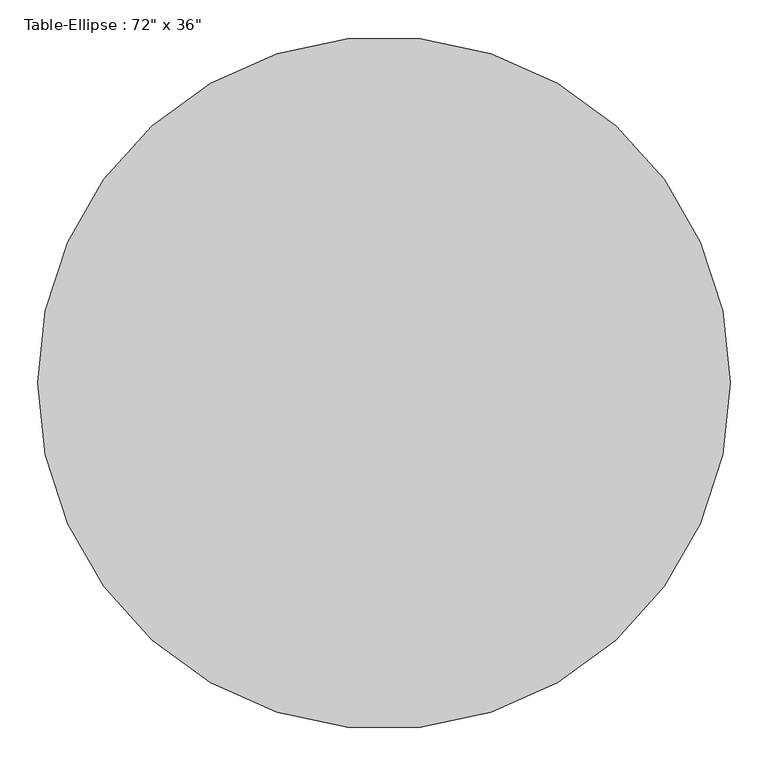
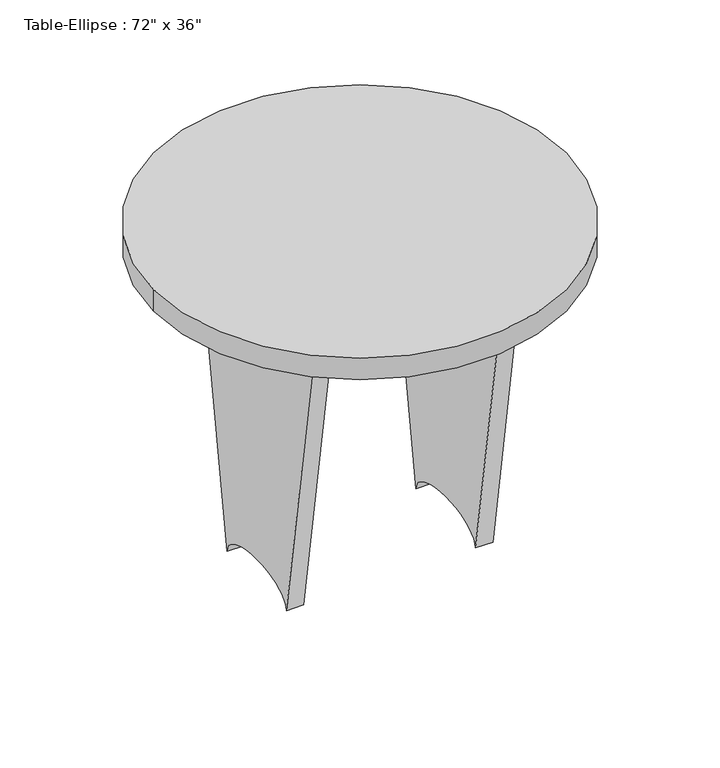
"""IFC4 building model written with IfcOpenShell, lengths in millimetres: furniture geometry."""

from ifc_helpers import new_model, si_unit, point, frame, origin, place, context, project, spatial, circle_curve, ellipse_curve, trimmed, source, transform, mapped, element, save
from ifc_brep_helpers import plane_surface, extruded_surface, advanced_brep


def furniture_4bee3317(model_context):
    return source(origin(), model_context, "Body", "AdvancedBrep", [
        advanced_brep(
        [(-190.5, 19.05, 711.2), (190.5, 19.05, 711.2), (190.5, 19.05, 474.1333333), (-190.5, 19.05, 474.1333333), (-190.5, -19.05, 711.2), (-190.5, -19.05, 474.1333333), (190.5, -19.05, 474.1333333), (190.5, -19.05, 711.2)],
        [
            (0, 1),
            (1, 2),
            (2, 3, ellipse_curve(frame((0.0, 19.05, 474.1333333), z_axis=(0.0, -1.0, 0.0), x_axis=(1.0, 0.0, 0.0)), 190.5, 101.6)),
            (3, 0),
            (4, 5),
            (5, 6, ellipse_curve(frame((0.0, -19.05, 474.1333333), z_axis=(0.0, 1.0, 0.0), x_axis=(1.0, 0.0, 0.0)), 190.5, 101.6)),
            (6, 7),
            (7, 4),
            (0, 4),
            (7, 1),
            (6, 2),
            (5, 3),
        ],
        [
            plane_surface(frame((-190.5, 19.05, 711.2), z_axis=(0.0, 1.0, 0.0), x_axis=(1.0, 0.0, 0.0))),
            plane_surface(frame((-190.5, -19.05, 711.2), z_axis=(0.0, -1.0, 0.0), x_axis=(-1.0, 0.0, 0.0))),
            plane_surface(frame((-190.5, 19.05, 711.2), z_axis=(0.0, 0.0, 1.0), x_axis=(0.0, -1.0, 0.0))),
            plane_surface(frame((190.5, 19.05, 711.2), z_axis=(1.0, 0.0, 0.0), x_axis=(0.0, -1.0, 0.0))),
            extruded_surface(trimmed(ellipse_curve(frame((0.0, -57.15, 474.1333333), z_axis=(0.0, -1.0, 0.0), x_axis=(1.0, 0.0, 0.0)), 190.5, 101.6), [point((190.5, -57.15, 474.1333333))], [point((-190.5, -57.15, 474.1333333))], True, "CARTESIAN"), (0.0, 38.099999999999994, 0.0), 38.099999999999994),
            plane_surface(frame((-190.5, 19.05, 474.1333333), z_axis=(-1.0, 0.0, 0.0), x_axis=(0.0, -1.0, 0.0))),
        ],
        [
            (0, [[1, 2, 3, 4]]),
            (1, [[5, 6, 7, 8]]),
            (2, [[-1, 9, -8, 10]]),
            (3, [[-2, -10, -7, 11]]),
            (4, [[-3, -11, -6, 12]]),
            (5, [[-4, -12, -5, -9]]),
        ],
    ),
        advanced_brep(
        [(228.6, 228.6, 711.2), (228.6, -228.6, 711.2), (228.6, -114.3, 0.0), (228.6, 114.3, 0.0), (190.5, 228.6, 711.2), (190.5, 114.3, 0.0), (190.5, -114.3, 0.0), (190.5, -228.6, 711.2)],
        [
            (0, 1),
            (1, 2),
            (2, 3, ellipse_curve(frame((228.6, 0.0, 0.0), z_axis=(-1.0, 0.0, 0.0), x_axis=(0.0, 1.0, 0.0)), 114.3, 50.8)),
            (3, 0),
            (4, 5),
            (5, 6, ellipse_curve(frame((190.5, 0.0, 0.0), z_axis=(1.0, 0.0, 0.0), x_axis=(0.0, 1.0, 0.0)), 114.3, 50.8)),
            (6, 7),
            (7, 4),
            (0, 4),
            (7, 1),
            (6, 2),
            (5, 3),
        ],
        [
            plane_surface(frame((228.6, -228.6, 711.2), z_axis=(1.0, 0.0, 0.0), x_axis=(0.0, -1.0, 0.0))),
            plane_surface(frame((190.5, -228.6, 711.2), z_axis=(-1.0, 0.0, 0.0), x_axis=(0.0, 1.0, 0.0))),
            plane_surface(frame((228.6, 228.6, 711.2), z_axis=(0.0, 0.0, 1.0), x_axis=(-1.0, 0.0, 0.0))),
            plane_surface(frame((228.6, -228.6, 711.2), z_axis=(0.0, -0.9873303712766982, -0.158678095383759), x_axis=(-1.0, 0.0, 0.0))),
            extruded_surface(trimmed(ellipse_curve(frame((152.4, 0.0, 0.0), z_axis=(-1.0, 0.0, 0.0), x_axis=(0.0, 1.0, 0.0)), 114.3, 50.8), [point((152.4, -114.3, 0.0))], [point((152.4, 114.3, 0.0))], True, "CARTESIAN"), (38.099999999999994, 0.0, 0.0), 38.099999999999994),
            plane_surface(frame((228.6, 114.3, 0.0), z_axis=(0.0, 0.9873303712767002, -0.15867809538374666), x_axis=(-1.0, 0.0, 0.0))),
        ],
        [
            (0, [[1, 2, 3, 4]]),
            (1, [[5, 6, 7, 8]]),
            (2, [[-1, 9, -8, 10]]),
            (3, [[-2, -10, -7, 11]]),
            (4, [[-3, -11, -6, 12]]),
            (5, [[-4, -12, -5, -9]]),
        ],
    ),
        advanced_brep(
        [(-190.5, 228.6, 711.2), (-190.5, -228.6, 711.2), (-190.5, -114.3, 0.0), (-190.5, 114.3, 0.0), (-228.6, 228.6, 711.2), (-228.6, 114.3, 0.0), (-228.6, -114.3, 0.0), (-228.6, -228.6, 711.2)],
        [
            (0, 1),
            (1, 2),
            (2, 3, ellipse_curve(frame((-190.5, 0.0, 0.0), z_axis=(-1.0, 0.0, 0.0), x_axis=(0.0, 1.0, 0.0)), 114.3, 50.8)),
            (3, 0),
            (4, 5),
            (5, 6, ellipse_curve(frame((-228.6, 0.0, 0.0), z_axis=(1.0, 0.0, 0.0), x_axis=(0.0, 1.0, 0.0)), 114.3, 50.8)),
            (6, 7),
            (7, 4),
            (0, 4),
            (7, 1),
            (6, 2),
            (5, 3),
        ],
        [
            plane_surface(frame((-190.5, -228.6, 711.2), z_axis=(1.0, 0.0, 0.0), x_axis=(0.0, -1.0, 0.0))),
            plane_surface(frame((-228.6, -228.6, 711.2), z_axis=(-1.0, 0.0, 0.0), x_axis=(0.0, 1.0, 0.0))),
            plane_surface(frame((-190.5, 228.6, 711.2), z_axis=(0.0, 0.0, 1.0), x_axis=(-1.0, 0.0, 0.0))),
            plane_surface(frame((-190.5, -228.6, 711.2), z_axis=(0.0, -0.9873303712766983, -0.15867809538375854), x_axis=(-1.0, 0.0, 0.0))),
            extruded_surface(trimmed(ellipse_curve(frame((-266.7, 0.0, 0.0), z_axis=(-1.0, 0.0, 0.0), x_axis=(0.0, 1.0, 0.0)), 114.3, 50.8), [point((-266.7, -114.3, 0.0))], [point((-266.7, 114.3, 0.0))], True, "CARTESIAN"), (38.099999999999994, 0.0, 0.0), 38.099999999999994),
            plane_surface(frame((-190.5, 114.3, 0.0), z_axis=(0.0, 0.9873303712766998, -0.15867809538374977), x_axis=(-1.0, 0.0, 0.0))),
        ],
        [
            (0, [[1, 2, 3, 4]]),
            (1, [[5, 6, 7, 8]]),
            (2, [[-1, 9, -8, 10]]),
            (3, [[-2, -10, -7, 11]]),
            (4, [[-3, -11, -6, 12]]),
            (5, [[-4, -12, -5, -9]]),
        ],
    ),
        advanced_brep(
        [(-457.2, 0.0, 762.0), (457.2, 0.0, 762.0), (-457.2, 0.0, 711.2), (457.2, 0.0, 711.2)],
        [
            (0, 1, circle_curve(frame((0.0, 0.0, 762.0), z_axis=(0.0, 0.0, 1.0), x_axis=(1.0, 0.0, 0.0)), 457.2)),
            (1, 0, circle_curve(frame((0.0, 0.0, 762.0), z_axis=(0.0, 0.0, 1.0), x_axis=(1.0, 0.0, 0.0)), 457.2)),
            (2, 3, ellipse_curve(frame((0.0, 0.0, 711.2), z_axis=(0.0, 0.0, -1.0), x_axis=(1.0, 0.0, 0.0)), 457.2, 457.2)),
            (3, 2, ellipse_curve(frame((0.0, 0.0, 711.2), z_axis=(0.0, 0.0, -1.0), x_axis=(1.0, 0.0, 0.0)), 457.2, 457.2)),
            (0, 2),
            (3, 1),
        ],
        [
            plane_surface(frame((457.2, 0.0, 762.0), z_axis=(0.0, 0.0, 1.0), x_axis=(0.0, 1.0, 0.0))),
            plane_surface(frame((457.2, 0.0, 711.2), z_axis=(0.0, 0.0, -1.0), x_axis=(0.0, -1.0, 0.0))),
            extruded_surface(trimmed(ellipse_curve(frame((0.0, 0.0, 660.4), z_axis=(0.0, 0.0, 1.0), x_axis=(1.0, 0.0, 0.0)), 457.2, 457.2), [point((-457.2, 0.0, 660.4))], [point((457.2, 0.0, 660.4))], True, "CARTESIAN"), (0.0, 0.0, 50.80000000000007), 50.80000000000007),
            extruded_surface(trimmed(ellipse_curve(frame((0.0, 0.0, 660.4), z_axis=(0.0, 0.0, 1.0), x_axis=(1.0, 0.0, 0.0)), 457.2, 457.2), [point((457.2, 0.0, 660.4))], [point((-457.2, 0.0, 660.4))], True, "CARTESIAN"), (0.0, 0.0, 50.80000000000007), 50.80000000000007),
        ],
        [
            (0, [[1, 2]]),
            (1, [[3, 4]]),
            (2, [[-1, 5, -4, 6]]),
            (3, [[-2, -6, -3, -5]]),
        ],
    ),
    ])


if __name__ == "__main__":
    model = new_model("IFC4")
    model_context = context("Model", 3, world=origin())
    ifc_project = project(units=[si_unit("LENGTHUNIT", "METRE", prefix="MILLI")], contexts=[model_context])
    site = spatial("IfcSite", under=ifc_project)
    building = spatial("IfcBuilding", under=site)
    placement = place(None, origin())
    furniture_shape = furniture_4bee3317(model_context)
    element("IfcFurniture", 1, ObjectType="Table-Ellipse : 72\" x 36\"", at=placement, inside=building, context=model_context, shape_type="MappedRepresentation", body=[
        mapped(furniture_shape, transform((0.0, 0.0, 0.0), x_axis=(1.0, 0.0, 0.0), y_axis=(0.0, 1.0, 0.0), z_axis=(0.0, 0.0, 1.0))),
    ])
    save(model, "model.ifc")

# Revit data of these elements
# Type "Table-Ellipse : 72\" x 36\""
#   Assembly Code = "E2020200"
#   Half Width = 1' - 6"
#   Half Length = 1' - 6"
#   Height = 2' - 6"
#   Length = 3' - 0"
#   Width = 3' - 0"
#   Base Material = Birch
#   Top Material = Laminate - Black
#   Default Elevation = 0
# Element 1 (IfcFurniture, "Table-Ellipse : 72\" x 36\"")
#   Materials on its faces: "Birch", "Laminate - Black"
# Materials
#   "Birch": class "Wood", colour RGB 210 159 95, transparency 0, Description = "Betula Alleghaniensis", Cost = 0
#   "Laminate - Black": colour RGB 0 0 0, transparency 0
